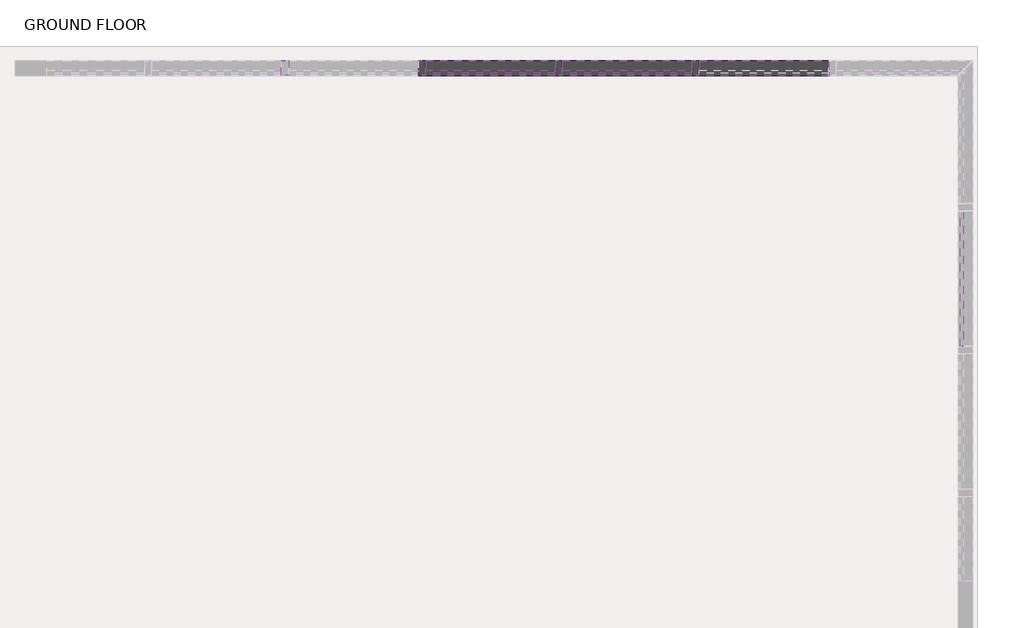
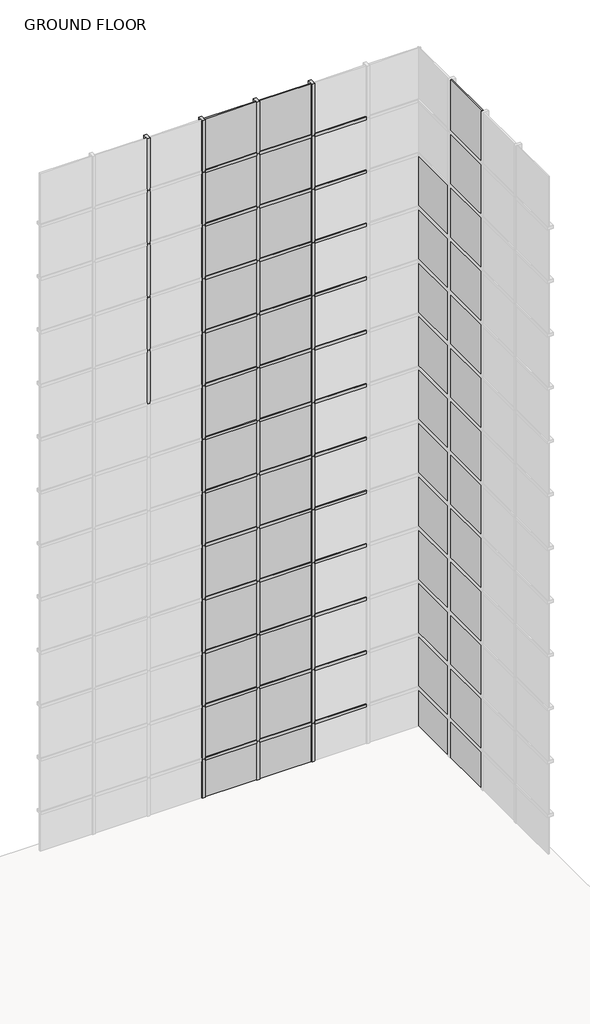
# One storey, part 13 of 16: 80 members, 50 plates.
"""IFC4 building model written with IfcOpenShell, lengths in millimetres."""

from ifc_helpers import new_model, si_unit, origin, place, context, project, spatial, transform, mapped, element, save
from components import member_d518c94e, member_b860638c, member_31fee25f, system_panel_glazed_5cba32e5, system_panel_glazed_49652e9e

model = new_model("IFC4")

# Units and contexts
model_context = context("Model", 3, world=origin())
ifc_project = project(units=[si_unit("LENGTHUNIT", "METRE", prefix="MILLI")], contexts=[model_context])

# Site, building, storey
site = spatial("IfcSite", under=ifc_project)
building = spatial("IfcBuilding", under=site)
storey = spatial("IfcBuildingStorey", under=building, Name="GROUND FLOOR", Elevation=0.0)

# Members
placement = place(None, origin())
member_shape = member_d518c94e(model_context)
element("IfcMember", 1, ObjectType="Rectangular Mullion : 2.5\" x 5\" rectangular", at=placement, inside=storey, context=model_context, shape_type="MappedRepresentation", body=[
    mapped(member_shape, transform((3695.2597848, 6370.2261968, 1168.8884615), x_axis=(0.0, 0.0, 1.0), y_axis=(0.0, 1.0, 0.0), z_axis=(-1.0, 0.0, 0.0))),
])
element("IfcMember", 2, ObjectType="Rectangular Mullion : 2.5\" x 5\" rectangular", at=placement, inside=storey, context=model_context, shape_type="MappedRepresentation", body=[
    mapped(member_shape, transform((2529.7905541, 6370.2261968, 1168.8884615), x_axis=(0.0, 0.0, 1.0), y_axis=(0.0, 1.0, 0.0), z_axis=(-1.0, 0.0, 0.0))),
])
element("IfcMember", 3, ObjectType="Rectangular Mullion : 2.5\" x 5\" rectangular", at=placement, inside=storey, context=model_context, shape_type="MappedRepresentation", body=[
    mapped(member_shape, transform((1364.3213234, 6370.2261968, 1168.8884615), x_axis=(0.0, 0.0, 1.0), y_axis=(0.0, 1.0, 0.0), z_axis=(-1.0, 0.0, 0.0))),
])
element("IfcMember", 4, ObjectType="Rectangular Mullion : 2.5\" x 5\" rectangular", at=placement, inside=storey, context=model_context, shape_type="MappedRepresentation", body=[
    mapped(member_shape, transform((3695.2597848, 6370.2261968, 2369.5269231), x_axis=(0.0, 0.0, 1.0), y_axis=(0.0, 1.0, 0.0), z_axis=(-1.0, 0.0, 0.0))),
])
element("IfcMember", 5, ObjectType="Rectangular Mullion : 2.5\" x 5\" rectangular", at=placement, inside=storey, context=model_context, shape_type="MappedRepresentation", body=[
    mapped(member_shape, transform((2529.7905541, 6370.2261968, 2369.5269231), x_axis=(0.0, 0.0, 1.0), y_axis=(0.0, 1.0, 0.0), z_axis=(-1.0, 0.0, 0.0))),
])
element("IfcMember", 6, ObjectType="Rectangular Mullion : 2.5\" x 5\" rectangular", at=placement, inside=storey, context=model_context, shape_type="MappedRepresentation", body=[
    mapped(member_shape, transform((1364.3213234, 6370.2261968, 2369.5269231), x_axis=(0.0, 0.0, 1.0), y_axis=(0.0, 1.0, 0.0), z_axis=(-1.0, 0.0, 0.0))),
])
element("IfcMember", 7, ObjectType="Rectangular Mullion : 2.5\" x 5\" rectangular", at=placement, inside=storey, context=model_context, shape_type="MappedRepresentation", body=[
    mapped(member_shape, transform((3695.2597848, 6370.2261968, 3570.1653846), x_axis=(0.0, 0.0, 1.0), y_axis=(0.0, 1.0, 0.0), z_axis=(-1.0, 0.0, 0.0))),
])
element("IfcMember", 8, ObjectType="Rectangular Mullion : 2.5\" x 5\" rectangular", at=placement, inside=storey, context=model_context, shape_type="MappedRepresentation", body=[
    mapped(member_shape, transform((2529.7905541, 6370.2261968, 3570.1653846), x_axis=(0.0, 0.0, 1.0), y_axis=(0.0, 1.0, 0.0), z_axis=(-1.0, 0.0, 0.0))),
])
element("IfcMember", 9, ObjectType="Rectangular Mullion : 2.5\" x 5\" rectangular", at=placement, inside=storey, context=model_context, shape_type="MappedRepresentation", body=[
    mapped(member_shape, transform((1364.3213234, 6370.2261968, 3570.1653846), x_axis=(0.0, 0.0, 1.0), y_axis=(0.0, 1.0, 0.0), z_axis=(-1.0, 0.0, 0.0))),
])
element("IfcMember", 10, ObjectType="Rectangular Mullion : 2.5\" x 5\" rectangular", at=placement, inside=storey, context=model_context, shape_type="MappedRepresentation", body=[
    mapped(member_shape, transform((3695.2597848, 6370.2261968, 4770.8038462), x_axis=(0.0, 0.0, 1.0), y_axis=(0.0, 1.0, 0.0), z_axis=(-1.0, 0.0, 0.0))),
])
element("IfcMember", 11, ObjectType="Rectangular Mullion : 2.5\" x 5\" rectangular", at=placement, inside=storey, context=model_context, shape_type="MappedRepresentation", body=[
    mapped(member_shape, transform((2529.7905541, 6370.2261968, 4770.8038462), x_axis=(0.0, 0.0, 1.0), y_axis=(0.0, 1.0, 0.0), z_axis=(-1.0, 0.0, 0.0))),
])
element("IfcMember", 12, ObjectType="Rectangular Mullion : 2.5\" x 5\" rectangular", at=placement, inside=storey, context=model_context, shape_type="MappedRepresentation", body=[
    mapped(member_shape, transform((1364.3213234, 6370.2261968, 4770.8038462), x_axis=(0.0, 0.0, 1.0), y_axis=(0.0, 1.0, 0.0), z_axis=(-1.0, 0.0, 0.0))),
])
element("IfcMember", 13, ObjectType="Rectangular Mullion : 2.5\" x 5\" rectangular", at=placement, inside=storey, context=model_context, shape_type="MappedRepresentation", body=[
    mapped(member_shape, transform((3695.2597848, 6370.2261968, 5971.4423077), x_axis=(0.0, 0.0, 1.0), y_axis=(0.0, 1.0, 0.0), z_axis=(-1.0, 0.0, 0.0))),
])
element("IfcMember", 14, ObjectType="Rectangular Mullion : 2.5\" x 5\" rectangular", at=placement, inside=storey, context=model_context, shape_type="MappedRepresentation", body=[
    mapped(member_shape, transform((2529.7905541, 6370.2261968, 5971.4423077), x_axis=(0.0, 0.0, 1.0), y_axis=(0.0, 1.0, 0.0), z_axis=(-1.0, 0.0, 0.0))),
])
element("IfcMember", 15, ObjectType="Rectangular Mullion : 2.5\" x 5\" rectangular", at=placement, inside=storey, context=model_context, shape_type="MappedRepresentation", body=[
    mapped(member_shape, transform((1364.3213234, 6370.2261968, 5971.4423077), x_axis=(0.0, 0.0, 1.0), y_axis=(0.0, 1.0, 0.0), z_axis=(-1.0, 0.0, 0.0))),
])
element("IfcMember", 16, ObjectType="Rectangular Mullion : 2.5\" x 5\" rectangular", at=placement, inside=storey, context=model_context, shape_type="MappedRepresentation", body=[
    mapped(member_shape, transform((3695.2597848, 6370.2261968, 7172.0807692), x_axis=(0.0, 0.0, 1.0), y_axis=(0.0, 1.0, 0.0), z_axis=(-1.0, 0.0, 0.0))),
])
element("IfcMember", 17, ObjectType="Rectangular Mullion : 2.5\" x 5\" rectangular", at=placement, inside=storey, context=model_context, shape_type="MappedRepresentation", body=[
    mapped(member_shape, transform((2529.7905541, 6370.2261968, 7172.0807692), x_axis=(0.0, 0.0, 1.0), y_axis=(0.0, 1.0, 0.0), z_axis=(-1.0, 0.0, 0.0))),
])
element("IfcMember", 18, ObjectType="Rectangular Mullion : 2.5\" x 5\" rectangular", at=placement, inside=storey, context=model_context, shape_type="MappedRepresentation", body=[
    mapped(member_shape, transform((1364.3213234, 6370.2261968, 7172.0807692), x_axis=(0.0, 0.0, 1.0), y_axis=(0.0, 1.0, 0.0), z_axis=(-1.0, 0.0, 0.0))),
])
element("IfcMember", 19, ObjectType="Rectangular Mullion : 2.5\" x 5\" rectangular", at=placement, inside=storey, context=model_context, shape_type="MappedRepresentation", body=[
    mapped(member_shape, transform((3695.2597848, 6370.2261968, 8372.7192308), x_axis=(0.0, 0.0, 1.0), y_axis=(0.0, 1.0, 0.0), z_axis=(-1.0, 0.0, 0.0))),
])
element("IfcMember", 20, ObjectType="Rectangular Mullion : 2.5\" x 5\" rectangular", at=placement, inside=storey, context=model_context, shape_type="MappedRepresentation", body=[
    mapped(member_shape, transform((2529.7905541, 6370.2261968, 8372.7192308), x_axis=(0.0, 0.0, 1.0), y_axis=(0.0, 1.0, 0.0), z_axis=(-1.0, 0.0, 0.0))),
])
element("IfcMember", 21, ObjectType="Rectangular Mullion : 2.5\" x 5\" rectangular", at=placement, inside=storey, context=model_context, shape_type="MappedRepresentation", body=[
    mapped(member_shape, transform((1364.3213234, 6370.2261968, 8372.7192308), x_axis=(0.0, 0.0, 1.0), y_axis=(0.0, 1.0, 0.0), z_axis=(-1.0, 0.0, 0.0))),
])
element("IfcMember", 22, ObjectType="Rectangular Mullion : 2.5\" x 5\" rectangular", at=placement, inside=storey, context=model_context, shape_type="MappedRepresentation", body=[
    mapped(member_shape, transform((3695.2597848, 6370.2261968, 9573.3576923), x_axis=(0.0, 0.0, 1.0), y_axis=(0.0, 1.0, 0.0), z_axis=(-1.0, 0.0, 0.0))),
])
element("IfcMember", 23, ObjectType="Rectangular Mullion : 2.5\" x 5\" rectangular", at=placement, inside=storey, context=model_context, shape_type="MappedRepresentation", body=[
    mapped(member_shape, transform((2529.7905541, 6370.2261968, 9573.3576923), x_axis=(0.0, 0.0, 1.0), y_axis=(0.0, 1.0, 0.0), z_axis=(-1.0, 0.0, 0.0))),
])
element("IfcMember", 24, ObjectType="Rectangular Mullion : 2.5\" x 5\" rectangular", at=placement, inside=storey, context=model_context, shape_type="MappedRepresentation", body=[
    mapped(member_shape, transform((1364.3213234, 6370.2261968, 9573.3576923), x_axis=(0.0, 0.0, 1.0), y_axis=(0.0, 1.0, 0.0), z_axis=(-1.0, 0.0, 0.0))),
])
element("IfcMember", 25, ObjectType="Rectangular Mullion : 2.5\" x 5\" rectangular", at=placement, inside=storey, context=model_context, shape_type="MappedRepresentation", body=[
    mapped(member_shape, transform((3695.2597848, 6370.2261968, 10773.9961538), x_axis=(0.0, 0.0, 1.0), y_axis=(0.0, 1.0, 0.0), z_axis=(-1.0, 0.0, 0.0))),
])
element("IfcMember", 26, ObjectType="Rectangular Mullion : 2.5\" x 5\" rectangular", at=placement, inside=storey, context=model_context, shape_type="MappedRepresentation", body=[
    mapped(member_shape, transform((2529.7905541, 6370.2261968, 10773.9961538), x_axis=(0.0, 0.0, 1.0), y_axis=(0.0, 1.0, 0.0), z_axis=(-1.0, 0.0, 0.0))),
])
element("IfcMember", 27, ObjectType="Rectangular Mullion : 2.5\" x 5\" rectangular", at=placement, inside=storey, context=model_context, shape_type="MappedRepresentation", body=[
    mapped(member_shape, transform((1364.3213234, 6370.2261968, 10773.9961538), x_axis=(0.0, 0.0, 1.0), y_axis=(0.0, 1.0, 0.0), z_axis=(-1.0, 0.0, 0.0))),
])
element("IfcMember", 28, ObjectType="Rectangular Mullion : 2.5\" x 5\" rectangular", at=placement, inside=storey, context=model_context, shape_type="MappedRepresentation", body=[
    mapped(member_shape, transform((3695.2597848, 6370.2261968, 11974.6346154), x_axis=(0.0, 0.0, 1.0), y_axis=(0.0, 1.0, 0.0), z_axis=(-1.0, 0.0, 0.0))),
])
element("IfcMember", 29, ObjectType="Rectangular Mullion : 2.5\" x 5\" rectangular", at=placement, inside=storey, context=model_context, shape_type="MappedRepresentation", body=[
    mapped(member_shape, transform((2529.7905541, 6370.2261968, 11974.6346154), x_axis=(0.0, 0.0, 1.0), y_axis=(0.0, 1.0, 0.0), z_axis=(-1.0, 0.0, 0.0))),
])
element("IfcMember", 30, ObjectType="Rectangular Mullion : 2.5\" x 5\" rectangular", at=placement, inside=storey, context=model_context, shape_type="MappedRepresentation", body=[
    mapped(member_shape, transform((1364.3213234, 6370.2261968, 11974.6346154), x_axis=(0.0, 0.0, 1.0), y_axis=(0.0, 1.0, 0.0), z_axis=(-1.0, 0.0, 0.0))),
])
element("IfcMember", 31, ObjectType="Rectangular Mullion : 2.5\" x 5\" rectangular", at=placement, inside=storey, context=model_context, shape_type="MappedRepresentation", body=[
    mapped(member_shape, transform((3695.2597848, 6370.2261968, 13175.2730769), x_axis=(0.0, 0.0, 1.0), y_axis=(0.0, 1.0, 0.0), z_axis=(-1.0, 0.0, 0.0))),
])
element("IfcMember", 32, ObjectType="Rectangular Mullion : 2.5\" x 5\" rectangular", at=placement, inside=storey, context=model_context, shape_type="MappedRepresentation", body=[
    mapped(member_shape, transform((2529.7905541, 6370.2261968, 13175.2730769), x_axis=(0.0, 0.0, 1.0), y_axis=(0.0, 1.0, 0.0), z_axis=(-1.0, 0.0, 0.0))),
])
element("IfcMember", 33, ObjectType="Rectangular Mullion : 2.5\" x 5\" rectangular", at=placement, inside=storey, context=model_context, shape_type="MappedRepresentation", body=[
    mapped(member_shape, transform((1364.3213234, 6370.2261968, 13175.2730769), x_axis=(0.0, 0.0, 1.0), y_axis=(0.0, 1.0, 0.0), z_axis=(-1.0, 0.0, 0.0))),
])
element("IfcMember", 34, ObjectType="Rectangular Mullion : 2.5\" x 5\" rectangular", at=placement, inside=storey, context=model_context, shape_type="MappedRepresentation", body=[
    mapped(member_shape, transform((3695.2597848, 6370.2261968, 14375.9115385), x_axis=(0.0, 0.0, 1.0), y_axis=(0.0, 1.0, 0.0), z_axis=(-1.0, 0.0, 0.0))),
])
element("IfcMember", 35, ObjectType="Rectangular Mullion : 2.5\" x 5\" rectangular", at=placement, inside=storey, context=model_context, shape_type="MappedRepresentation", body=[
    mapped(member_shape, transform((2529.7905541, 6370.2261968, 14375.9115385), x_axis=(0.0, 0.0, 1.0), y_axis=(0.0, 1.0, 0.0), z_axis=(-1.0, 0.0, 0.0))),
])
element("IfcMember", 36, ObjectType="Rectangular Mullion : 2.5\" x 5\" rectangular", at=placement, inside=storey, context=model_context, shape_type="MappedRepresentation", body=[
    mapped(member_shape, transform((1364.3213234, 6370.2261968, 14375.9115385), x_axis=(0.0, 0.0, 1.0), y_axis=(0.0, 1.0, 0.0), z_axis=(-1.0, 0.0, 0.0))),
])
member_2_shape = member_b860638c(model_context)
element("IfcMember", 37, ObjectType="Rectangular Mullion : 2.5\" x 5\" rectangular", at=placement, inside=storey, context=model_context, shape_type="MappedRepresentation", body=[
    mapped(member_2_shape, transform((3663.5097848, 6370.2261968, 0.0), x_axis=(-1.0, 0.0, 0.0), y_axis=(0.0, 1.0, 0.0), z_axis=(0.0, 0.0, -1.0))),
])
element("IfcMember", 38, ObjectType="Rectangular Mullion : 2.5\" x 5\" rectangular", at=placement, inside=storey, context=model_context, shape_type="MappedRepresentation", body=[
    mapped(member_2_shape, transform((2498.0405541, 6370.2261968, 0.0), x_axis=(-1.0, 0.0, 0.0), y_axis=(0.0, 1.0, 0.0), z_axis=(0.0, 0.0, -1.0))),
])
element("IfcMember", 39, ObjectType="Rectangular Mullion : 2.5\" x 5\" rectangular", at=placement, inside=storey, context=model_context, shape_type="MappedRepresentation", body=[
    mapped(member_2_shape, transform((1332.5713234, 6370.2261968, 0.0), x_axis=(-1.0, 0.0, 0.0), y_axis=(0.0, 1.0, 0.0), z_axis=(0.0, 0.0, -1.0))),
])
member_3_shape = member_31fee25f(model_context)
element("IfcMember", 40, ObjectType="Rectangular Mullion : 2.5\" x 5\" rectangular", at=placement, inside=storey, context=model_context, shape_type="MappedRepresentation", body=[
    mapped(member_3_shape, transform((3663.5097848, 6370.2261968, 1168.8884615), x_axis=(-1.0, 0.0, 0.0), y_axis=(0.0, 1.0, 0.0), z_axis=(0.0, 0.0, -1.0))),
])
element("IfcMember", 41, ObjectType="Rectangular Mullion : 2.5\" x 5\" rectangular", at=placement, inside=storey, context=model_context, shape_type="MappedRepresentation", body=[
    mapped(member_3_shape, transform((2498.0405541, 6370.2261968, 1168.8884615), x_axis=(-1.0, 0.0, 0.0), y_axis=(0.0, 1.0, 0.0), z_axis=(0.0, 0.0, -1.0))),
])
element("IfcMember", 42, ObjectType="Rectangular Mullion : 2.5\" x 5\" rectangular", at=placement, inside=storey, context=model_context, shape_type="MappedRepresentation", body=[
    mapped(member_3_shape, transform((1332.5713234, 6370.2261968, 1168.8884615), x_axis=(-1.0, 0.0, 0.0), y_axis=(0.0, 1.0, 0.0), z_axis=(0.0, 0.0, -1.0))),
])
element("IfcMember", 43, ObjectType="Rectangular Mullion : 2.5\" x 5\" rectangular", at=placement, inside=storey, context=model_context, shape_type="MappedRepresentation", body=[
    mapped(member_3_shape, transform((3663.5097848, 6370.2261968, 2369.5269231), x_axis=(-1.0, 0.0, 0.0), y_axis=(0.0, 1.0, 0.0), z_axis=(0.0, 0.0, -1.0))),
])
element("IfcMember", 44, ObjectType="Rectangular Mullion : 2.5\" x 5\" rectangular", at=placement, inside=storey, context=model_context, shape_type="MappedRepresentation", body=[
    mapped(member_3_shape, transform((2498.0405541, 6370.2261968, 2369.5269231), x_axis=(-1.0, 0.0, 0.0), y_axis=(0.0, 1.0, 0.0), z_axis=(0.0, 0.0, -1.0))),
])
element("IfcMember", 45, ObjectType="Rectangular Mullion : 2.5\" x 5\" rectangular", at=placement, inside=storey, context=model_context, shape_type="MappedRepresentation", body=[
    mapped(member_3_shape, transform((1332.5713234, 6370.2261968, 2369.5269231), x_axis=(-1.0, 0.0, 0.0), y_axis=(0.0, 1.0, 0.0), z_axis=(0.0, 0.0, -1.0))),
])
element("IfcMember", 46, ObjectType="Rectangular Mullion : 2.5\" x 5\" rectangular", at=placement, inside=storey, context=model_context, shape_type="MappedRepresentation", body=[
    mapped(member_3_shape, transform((3663.5097848, 6370.2261968, 3570.1653846), x_axis=(-1.0, 0.0, 0.0), y_axis=(0.0, 1.0, 0.0), z_axis=(0.0, 0.0, -1.0))),
])
element("IfcMember", 47, ObjectType="Rectangular Mullion : 2.5\" x 5\" rectangular", at=placement, inside=storey, context=model_context, shape_type="MappedRepresentation", body=[
    mapped(member_3_shape, transform((2498.0405541, 6370.2261968, 3570.1653846), x_axis=(-1.0, 0.0, 0.0), y_axis=(0.0, 1.0, 0.0), z_axis=(0.0, 0.0, -1.0))),
])
element("IfcMember", 48, ObjectType="Rectangular Mullion : 2.5\" x 5\" rectangular", at=placement, inside=storey, context=model_context, shape_type="MappedRepresentation", body=[
    mapped(member_3_shape, transform((1332.5713234, 6370.2261968, 3570.1653846), x_axis=(-1.0, 0.0, 0.0), y_axis=(0.0, 1.0, 0.0), z_axis=(0.0, 0.0, -1.0))),
])
element("IfcMember", 49, ObjectType="Rectangular Mullion : 2.5\" x 5\" rectangular", at=placement, inside=storey, context=model_context, shape_type="MappedRepresentation", body=[
    mapped(member_3_shape, transform((3663.5097848, 6370.2261968, 4770.8038462), x_axis=(-1.0, 0.0, 0.0), y_axis=(0.0, 1.0, 0.0), z_axis=(0.0, 0.0, -1.0))),
])
element("IfcMember", 50, ObjectType="Rectangular Mullion : 2.5\" x 5\" rectangular", at=placement, inside=storey, context=model_context, shape_type="MappedRepresentation", body=[
    mapped(member_3_shape, transform((2498.0405541, 6370.2261968, 4770.8038462), x_axis=(-1.0, 0.0, 0.0), y_axis=(0.0, 1.0, 0.0), z_axis=(0.0, 0.0, -1.0))),
])
element("IfcMember", 51, ObjectType="Rectangular Mullion : 2.5\" x 5\" rectangular", at=placement, inside=storey, context=model_context, shape_type="MappedRepresentation", body=[
    mapped(member_3_shape, transform((1332.5713234, 6370.2261968, 4770.8038462), x_axis=(-1.0, 0.0, 0.0), y_axis=(0.0, 1.0, 0.0), z_axis=(0.0, 0.0, -1.0))),
])
element("IfcMember", 52, ObjectType="Rectangular Mullion : 2.5\" x 5\" rectangular", at=placement, inside=storey, context=model_context, shape_type="MappedRepresentation", body=[
    mapped(member_3_shape, transform((3663.5097848, 6370.2261968, 5971.4423077), x_axis=(-1.0, 0.0, 0.0), y_axis=(0.0, 1.0, 0.0), z_axis=(0.0, 0.0, -1.0))),
])
element("IfcMember", 53, ObjectType="Rectangular Mullion : 2.5\" x 5\" rectangular", at=placement, inside=storey, context=model_context, shape_type="MappedRepresentation", body=[
    mapped(member_3_shape, transform((2498.0405541, 6370.2261968, 5971.4423077), x_axis=(-1.0, 0.0, 0.0), y_axis=(0.0, 1.0, 0.0), z_axis=(0.0, 0.0, -1.0))),
])
element("IfcMember", 54, ObjectType="Rectangular Mullion : 2.5\" x 5\" rectangular", at=placement, inside=storey, context=model_context, shape_type="MappedRepresentation", body=[
    mapped(member_3_shape, transform((1332.5713234, 6370.2261968, 5971.4423077), x_axis=(-1.0, 0.0, 0.0), y_axis=(0.0, 1.0, 0.0), z_axis=(0.0, 0.0, -1.0))),
])
element("IfcMember", 55, ObjectType="Rectangular Mullion : 2.5\" x 5\" rectangular", at=placement, inside=storey, context=model_context, shape_type="MappedRepresentation", body=[
    mapped(member_3_shape, transform((3663.5097848, 6370.2261968, 7172.0807692), x_axis=(-1.0, 0.0, 0.0), y_axis=(0.0, 1.0, 0.0), z_axis=(0.0, 0.0, -1.0))),
])
element("IfcMember", 56, ObjectType="Rectangular Mullion : 2.5\" x 5\" rectangular", at=placement, inside=storey, context=model_context, shape_type="MappedRepresentation", body=[
    mapped(member_3_shape, transform((2498.0405541, 6370.2261968, 7172.0807692), x_axis=(-1.0, 0.0, 0.0), y_axis=(0.0, 1.0, 0.0), z_axis=(0.0, 0.0, -1.0))),
])
element("IfcMember", 57, ObjectType="Rectangular Mullion : 2.5\" x 5\" rectangular", at=placement, inside=storey, context=model_context, shape_type="MappedRepresentation", body=[
    mapped(member_3_shape, transform((1332.5713234, 6370.2261968, 7172.0807692), x_axis=(-1.0, 0.0, 0.0), y_axis=(0.0, 1.0, 0.0), z_axis=(0.0, 0.0, -1.0))),
])
element("IfcMember", 58, ObjectType="Rectangular Mullion : 2.5\" x 5\" rectangular", at=placement, inside=storey, context=model_context, shape_type="MappedRepresentation", body=[
    mapped(member_3_shape, transform((3663.5097848, 6370.2261968, 8372.7192308), x_axis=(-1.0, 0.0, 0.0), y_axis=(0.0, 1.0, 0.0), z_axis=(0.0, 0.0, -1.0))),
])
element("IfcMember", 59, ObjectType="Rectangular Mullion : 2.5\" x 5\" rectangular", at=placement, inside=storey, context=model_context, shape_type="MappedRepresentation", body=[
    mapped(member_3_shape, transform((2498.0405541, 6370.2261968, 8372.7192308), x_axis=(-1.0, 0.0, 0.0), y_axis=(0.0, 1.0, 0.0), z_axis=(0.0, 0.0, -1.0))),
])
element("IfcMember", 60, ObjectType="Rectangular Mullion : 2.5\" x 5\" rectangular", at=placement, inside=storey, context=model_context, shape_type="MappedRepresentation", body=[
    mapped(member_3_shape, transform((1332.5713234, 6370.2261968, 8372.7192308), x_axis=(-1.0, 0.0, 0.0), y_axis=(0.0, 1.0, 0.0), z_axis=(0.0, 0.0, -1.0))),
])
element("IfcMember", 61, ObjectType="Rectangular Mullion : 2.5\" x 5\" rectangular", at=placement, inside=storey, context=model_context, shape_type="MappedRepresentation", body=[
    mapped(member_3_shape, transform((3663.5097848, 6370.2261968, 9573.3576923), x_axis=(-1.0, 0.0, 0.0), y_axis=(0.0, 1.0, 0.0), z_axis=(0.0, 0.0, -1.0))),
])
element("IfcMember", 62, ObjectType="Rectangular Mullion : 2.5\" x 5\" rectangular", at=placement, inside=storey, context=model_context, shape_type="MappedRepresentation", body=[
    mapped(member_3_shape, transform((2498.0405541, 6370.2261968, 9573.3576923), x_axis=(-1.0, 0.0, 0.0), y_axis=(0.0, 1.0, 0.0), z_axis=(0.0, 0.0, -1.0))),
])
element("IfcMember", 63, ObjectType="Rectangular Mullion : 2.5\" x 5\" rectangular", at=placement, inside=storey, context=model_context, shape_type="MappedRepresentation", body=[
    mapped(member_3_shape, transform((1332.5713234, 6370.2261968, 9573.3576923), x_axis=(-1.0, 0.0, 0.0), y_axis=(0.0, 1.0, 0.0), z_axis=(0.0, 0.0, -1.0))),
])
element("IfcMember", 64, ObjectType="Rectangular Mullion : 2.5\" x 5\" rectangular", at=placement, inside=storey, context=model_context, shape_type="MappedRepresentation", body=[
    mapped(member_3_shape, transform((167.1020927, 6370.2261968, 9573.3576923), x_axis=(-1.0, 0.0, 0.0), y_axis=(0.0, 1.0, 0.0), z_axis=(0.0, 0.0, -1.0))),
])
element("IfcMember", 65, ObjectType="Rectangular Mullion : 2.5\" x 5\" rectangular", at=placement, inside=storey, context=model_context, shape_type="MappedRepresentation", body=[
    mapped(member_3_shape, transform((3663.5097848, 6370.2261968, 10773.9961538), x_axis=(-1.0, 0.0, 0.0), y_axis=(0.0, 1.0, 0.0), z_axis=(0.0, 0.0, -1.0))),
])
element("IfcMember", 66, ObjectType="Rectangular Mullion : 2.5\" x 5\" rectangular", at=placement, inside=storey, context=model_context, shape_type="MappedRepresentation", body=[
    mapped(member_3_shape, transform((2498.0405541, 6370.2261968, 10773.9961538), x_axis=(-1.0, 0.0, 0.0), y_axis=(0.0, 1.0, 0.0), z_axis=(0.0, 0.0, -1.0))),
])
element("IfcMember", 67, ObjectType="Rectangular Mullion : 2.5\" x 5\" rectangular", at=placement, inside=storey, context=model_context, shape_type="MappedRepresentation", body=[
    mapped(member_3_shape, transform((1332.5713234, 6370.2261968, 10773.9961538), x_axis=(-1.0, 0.0, 0.0), y_axis=(0.0, 1.0, 0.0), z_axis=(0.0, 0.0, -1.0))),
])
element("IfcMember", 68, ObjectType="Rectangular Mullion : 2.5\" x 5\" rectangular", at=placement, inside=storey, context=model_context, shape_type="MappedRepresentation", body=[
    mapped(member_3_shape, transform((167.1020927, 6370.2261968, 10773.9961538), x_axis=(-1.0, 0.0, 0.0), y_axis=(0.0, 1.0, 0.0), z_axis=(0.0, 0.0, -1.0))),
])
element("IfcMember", 69, ObjectType="Rectangular Mullion : 2.5\" x 5\" rectangular", at=placement, inside=storey, context=model_context, shape_type="MappedRepresentation", body=[
    mapped(member_3_shape, transform((3663.5097848, 6370.2261968, 11974.6346154), x_axis=(-1.0, 0.0, 0.0), y_axis=(0.0, 1.0, 0.0), z_axis=(0.0, 0.0, -1.0))),
])
element("IfcMember", 70, ObjectType="Rectangular Mullion : 2.5\" x 5\" rectangular", at=placement, inside=storey, context=model_context, shape_type="MappedRepresentation", body=[
    mapped(member_3_shape, transform((2498.0405541, 6370.2261968, 11974.6346154), x_axis=(-1.0, 0.0, 0.0), y_axis=(0.0, 1.0, 0.0), z_axis=(0.0, 0.0, -1.0))),
])
element("IfcMember", 71, ObjectType="Rectangular Mullion : 2.5\" x 5\" rectangular", at=placement, inside=storey, context=model_context, shape_type="MappedRepresentation", body=[
    mapped(member_3_shape, transform((1332.5713234, 6370.2261968, 11974.6346154), x_axis=(-1.0, 0.0, 0.0), y_axis=(0.0, 1.0, 0.0), z_axis=(0.0, 0.0, -1.0))),
])
element("IfcMember", 72, ObjectType="Rectangular Mullion : 2.5\" x 5\" rectangular", at=placement, inside=storey, context=model_context, shape_type="MappedRepresentation", body=[
    mapped(member_3_shape, transform((167.1020927, 6370.2261968, 11974.6346154), x_axis=(-1.0, 0.0, 0.0), y_axis=(0.0, 1.0, 0.0), z_axis=(0.0, 0.0, -1.0))),
])
element("IfcMember", 73, ObjectType="Rectangular Mullion : 2.5\" x 5\" rectangular", at=placement, inside=storey, context=model_context, shape_type="MappedRepresentation", body=[
    mapped(member_3_shape, transform((3663.5097848, 6370.2261968, 13175.2730769), x_axis=(-1.0, 0.0, 0.0), y_axis=(0.0, 1.0, 0.0), z_axis=(0.0, 0.0, -1.0))),
])
element("IfcMember", 74, ObjectType="Rectangular Mullion : 2.5\" x 5\" rectangular", at=placement, inside=storey, context=model_context, shape_type="MappedRepresentation", body=[
    mapped(member_3_shape, transform((2498.0405541, 6370.2261968, 13175.2730769), x_axis=(-1.0, 0.0, 0.0), y_axis=(0.0, 1.0, 0.0), z_axis=(0.0, 0.0, -1.0))),
])
element("IfcMember", 75, ObjectType="Rectangular Mullion : 2.5\" x 5\" rectangular", at=placement, inside=storey, context=model_context, shape_type="MappedRepresentation", body=[
    mapped(member_3_shape, transform((1332.5713234, 6370.2261968, 13175.2730769), x_axis=(-1.0, 0.0, 0.0), y_axis=(0.0, 1.0, 0.0), z_axis=(0.0, 0.0, -1.0))),
])
element("IfcMember", 76, ObjectType="Rectangular Mullion : 2.5\" x 5\" rectangular", at=placement, inside=storey, context=model_context, shape_type="MappedRepresentation", body=[
    mapped(member_3_shape, transform((167.1020927, 6370.2261968, 13175.2730769), x_axis=(-1.0, 0.0, 0.0), y_axis=(0.0, 1.0, 0.0), z_axis=(0.0, 0.0, -1.0))),
])
element("IfcMember", 77, ObjectType="Rectangular Mullion : 2.5\" x 5\" rectangular", at=placement, inside=storey, context=model_context, shape_type="MappedRepresentation", body=[
    mapped(member_2_shape, transform((3663.5097848, 6370.2261968, 14375.9115385), x_axis=(-1.0, 0.0, 0.0), y_axis=(0.0, 1.0, 0.0), z_axis=(0.0, 0.0, -1.0))),
])
element("IfcMember", 78, ObjectType="Rectangular Mullion : 2.5\" x 5\" rectangular", at=placement, inside=storey, context=model_context, shape_type="MappedRepresentation", body=[
    mapped(member_2_shape, transform((2498.0405541, 6370.2261968, 14375.9115385), x_axis=(-1.0, 0.0, 0.0), y_axis=(0.0, 1.0, 0.0), z_axis=(0.0, 0.0, -1.0))),
])
element("IfcMember", 79, ObjectType="Rectangular Mullion : 2.5\" x 5\" rectangular", at=placement, inside=storey, context=model_context, shape_type="MappedRepresentation", body=[
    mapped(member_2_shape, transform((1332.5713234, 6370.2261968, 14375.9115385), x_axis=(-1.0, 0.0, 0.0), y_axis=(0.0, 1.0, 0.0), z_axis=(0.0, 0.0, -1.0))),
])
element("IfcMember", 80, ObjectType="Rectangular Mullion : 2.5\" x 5\" rectangular", at=placement, inside=storey, context=model_context, shape_type="MappedRepresentation", body=[
    mapped(member_2_shape, transform((167.1020927, 6370.2261968, 14375.9115385), x_axis=(-1.0, 0.0, 0.0), y_axis=(0.0, 1.0, 0.0), z_axis=(0.0, 0.0, -1.0))),
])

# Plates
system_panel_glazed_shape = system_panel_glazed_5cba32e5(model_context)
element("IfcPlate", 81, ObjectType="System Panel : Glazed", at=placement, inside=storey, context=model_context, shape_type="MappedRepresentation", body=[
    mapped(system_panel_glazed_shape, transform((3080.7751695, 6370.2261968, 0.0), x_axis=(-1.0, 0.0, 0.0), y_axis=(0.0, -1.0, 0.0), z_axis=(0.0, 0.0, 1.0))),
])
element("IfcPlate", 82, ObjectType="System Panel : Glazed", at=placement, inside=storey, context=model_context, shape_type="MappedRepresentation", body=[
    mapped(system_panel_glazed_shape, transform((1915.3059387, 6370.2261968, 0.0), x_axis=(-1.0, 0.0, 0.0), y_axis=(0.0, -1.0, 0.0), z_axis=(0.0, 0.0, 1.0))),
])
element("IfcPlate", 83, ObjectType="System Panel : Glazed", at=placement, inside=storey, context=model_context, shape_type="MappedRepresentation", body=[
    mapped(system_panel_glazed_shape, transform((3080.7751695, 6370.2261968, 1200.6384615), x_axis=(-1.0, 0.0, 0.0), y_axis=(0.0, -1.0, 0.0), z_axis=(0.0, 0.0, 1.0))),
])
element("IfcPlate", 84, ObjectType="System Panel : Glazed", at=placement, inside=storey, context=model_context, shape_type="MappedRepresentation", body=[
    mapped(system_panel_glazed_shape, transform((1915.3059387, 6370.2261968, 1200.6384615), x_axis=(-1.0, 0.0, 0.0), y_axis=(0.0, -1.0, 0.0), z_axis=(0.0, 0.0, 1.0))),
])
element("IfcPlate", 85, ObjectType="System Panel : Glazed", at=placement, inside=storey, context=model_context, shape_type="MappedRepresentation", body=[
    mapped(system_panel_glazed_shape, transform((3080.7751695, 6370.2261968, 2401.2769231), x_axis=(-1.0, 0.0, 0.0), y_axis=(0.0, -1.0, 0.0), z_axis=(0.0, 0.0, 1.0))),
])
element("IfcPlate", 86, ObjectType="System Panel : Glazed", at=placement, inside=storey, context=model_context, shape_type="MappedRepresentation", body=[
    mapped(system_panel_glazed_shape, transform((1915.3059387, 6370.2261968, 2401.2769231), x_axis=(-1.0, 0.0, 0.0), y_axis=(0.0, -1.0, 0.0), z_axis=(0.0, 0.0, 1.0))),
])
element("IfcPlate", 87, ObjectType="System Panel : Glazed", at=placement, inside=storey, context=model_context, shape_type="MappedRepresentation", body=[
    mapped(system_panel_glazed_shape, transform((3080.7751695, 6370.2261968, 3601.9153846), x_axis=(-1.0, 0.0, 0.0), y_axis=(0.0, -1.0, 0.0), z_axis=(0.0, 0.0, 1.0))),
])
element("IfcPlate", 88, ObjectType="System Panel : Glazed", at=placement, inside=storey, context=model_context, shape_type="MappedRepresentation", body=[
    mapped(system_panel_glazed_shape, transform((1915.3059387, 6370.2261968, 3601.9153846), x_axis=(-1.0, 0.0, 0.0), y_axis=(0.0, -1.0, 0.0), z_axis=(0.0, 0.0, 1.0))),
])
element("IfcPlate", 89, ObjectType="System Panel : Glazed", at=placement, inside=storey, context=model_context, shape_type="MappedRepresentation", body=[
    mapped(system_panel_glazed_shape, transform((3080.7751695, 6370.2261968, 4802.5538462), x_axis=(-1.0, 0.0, 0.0), y_axis=(0.0, -1.0, 0.0), z_axis=(0.0, 0.0, 1.0))),
])
element("IfcPlate", 90, ObjectType="System Panel : Glazed", at=placement, inside=storey, context=model_context, shape_type="MappedRepresentation", body=[
    mapped(system_panel_glazed_shape, transform((1915.3059387, 6370.2261968, 4802.5538462), x_axis=(-1.0, 0.0, 0.0), y_axis=(0.0, -1.0, 0.0), z_axis=(0.0, 0.0, 1.0))),
])
element("IfcPlate", 91, ObjectType="System Panel : Glazed", at=placement, inside=storey, context=model_context, shape_type="MappedRepresentation", body=[
    mapped(system_panel_glazed_shape, transform((3080.7751695, 6370.2261968, 6003.1923077), x_axis=(-1.0, 0.0, 0.0), y_axis=(0.0, -1.0, 0.0), z_axis=(0.0, 0.0, 1.0))),
])
element("IfcPlate", 92, ObjectType="System Panel : Glazed", at=placement, inside=storey, context=model_context, shape_type="MappedRepresentation", body=[
    mapped(system_panel_glazed_shape, transform((1915.3059387, 6370.2261968, 6003.1923077), x_axis=(-1.0, 0.0, 0.0), y_axis=(0.0, -1.0, 0.0), z_axis=(0.0, 0.0, 1.0))),
])
element("IfcPlate", 93, ObjectType="System Panel : Glazed", at=placement, inside=storey, context=model_context, shape_type="MappedRepresentation", body=[
    mapped(system_panel_glazed_shape, transform((3080.7751695, 6370.2261968, 7203.8307692), x_axis=(-1.0, 0.0, 0.0), y_axis=(0.0, -1.0, 0.0), z_axis=(0.0, 0.0, 1.0))),
])
element("IfcPlate", 94, ObjectType="System Panel : Glazed", at=placement, inside=storey, context=model_context, shape_type="MappedRepresentation", body=[
    mapped(system_panel_glazed_shape, transform((1915.3059387, 6370.2261968, 7203.8307692), x_axis=(-1.0, 0.0, 0.0), y_axis=(0.0, -1.0, 0.0), z_axis=(0.0, 0.0, 1.0))),
])
element("IfcPlate", 95, ObjectType="System Panel : Glazed", at=placement, inside=storey, context=model_context, shape_type="MappedRepresentation", body=[
    mapped(system_panel_glazed_shape, transform((3080.7751695, 6370.2261968, 8404.4692308), x_axis=(-1.0, 0.0, 0.0), y_axis=(0.0, -1.0, 0.0), z_axis=(0.0, 0.0, 1.0))),
])
element("IfcPlate", 96, ObjectType="System Panel : Glazed", at=placement, inside=storey, context=model_context, shape_type="MappedRepresentation", body=[
    mapped(system_panel_glazed_shape, transform((1915.3059387, 6370.2261968, 8404.4692308), x_axis=(-1.0, 0.0, 0.0), y_axis=(0.0, -1.0, 0.0), z_axis=(0.0, 0.0, 1.0))),
])
element("IfcPlate", 97, ObjectType="System Panel : Glazed", at=placement, inside=storey, context=model_context, shape_type="MappedRepresentation", body=[
    mapped(system_panel_glazed_shape, transform((3080.7751695, 6370.2261968, 9605.1076923), x_axis=(-1.0, 0.0, 0.0), y_axis=(0.0, -1.0, 0.0), z_axis=(0.0, 0.0, 1.0))),
])
element("IfcPlate", 98, ObjectType="System Panel : Glazed", at=placement, inside=storey, context=model_context, shape_type="MappedRepresentation", body=[
    mapped(system_panel_glazed_shape, transform((1915.3059387, 6370.2261968, 9605.1076923), x_axis=(-1.0, 0.0, 0.0), y_axis=(0.0, -1.0, 0.0), z_axis=(0.0, 0.0, 1.0))),
])
element("IfcPlate", 99, ObjectType="System Panel : Glazed", at=placement, inside=storey, context=model_context, shape_type="MappedRepresentation", body=[
    mapped(system_panel_glazed_shape, transform((3080.7751695, 6370.2261968, 10805.7461538), x_axis=(-1.0, 0.0, 0.0), y_axis=(0.0, -1.0, 0.0), z_axis=(0.0, 0.0, 1.0))),
])
element("IfcPlate", 100, ObjectType="System Panel : Glazed", at=placement, inside=storey, context=model_context, shape_type="MappedRepresentation", body=[
    mapped(system_panel_glazed_shape, transform((1915.3059387, 6370.2261968, 10805.7461538), x_axis=(-1.0, 0.0, 0.0), y_axis=(0.0, -1.0, 0.0), z_axis=(0.0, 0.0, 1.0))),
])
element("IfcPlate", 101, ObjectType="System Panel : Glazed", at=placement, inside=storey, context=model_context, shape_type="MappedRepresentation", body=[
    mapped(system_panel_glazed_shape, transform((3080.7751695, 6370.2261968, 12006.3846154), x_axis=(-1.0, 0.0, 0.0), y_axis=(0.0, -1.0, 0.0), z_axis=(0.0, 0.0, 1.0))),
])
element("IfcPlate", 102, ObjectType="System Panel : Glazed", at=placement, inside=storey, context=model_context, shape_type="MappedRepresentation", body=[
    mapped(system_panel_glazed_shape, transform((1915.3059387, 6370.2261968, 12006.3846154), x_axis=(-1.0, 0.0, 0.0), y_axis=(0.0, -1.0, 0.0), z_axis=(0.0, 0.0, 1.0))),
])
element("IfcPlate", 103, ObjectType="System Panel : Glazed", at=placement, inside=storey, context=model_context, shape_type="MappedRepresentation", body=[
    mapped(system_panel_glazed_shape, transform((3080.7751695, 6370.2261968, 13207.0230769), x_axis=(-1.0, 0.0, 0.0), y_axis=(0.0, -1.0, 0.0), z_axis=(0.0, 0.0, 1.0))),
])
element("IfcPlate", 104, ObjectType="System Panel : Glazed", at=placement, inside=storey, context=model_context, shape_type="MappedRepresentation", body=[
    mapped(system_panel_glazed_shape, transform((1915.3059387, 6370.2261968, 13207.0230769), x_axis=(-1.0, 0.0, 0.0), y_axis=(0.0, -1.0, 0.0), z_axis=(0.0, 0.0, 1.0))),
])
element("IfcPlate", 105, ObjectType="System Panel : Glazed", at=placement, inside=storey, context=model_context, shape_type="MappedRepresentation", body=[
    mapped(system_panel_glazed_shape, transform((3080.7751695, 6370.2261968, 14407.6615385), x_axis=(-1.0, 0.0, 0.0), y_axis=(0.0, -1.0, 0.0), z_axis=(0.0, 0.0, 1.0))),
])
element("IfcPlate", 106, ObjectType="System Panel : Glazed", at=placement, inside=storey, context=model_context, shape_type="MappedRepresentation", body=[
    mapped(system_panel_glazed_shape, transform((1915.3059387, 6370.2261968, 14407.6615385), x_axis=(-1.0, 0.0, 0.0), y_axis=(0.0, -1.0, 0.0), z_axis=(0.0, 0.0, 1.0))),
])
system_panel_glazed_2_shape = system_panel_glazed_49652e9e(model_context)
element("IfcPlate", 107, ObjectType="System Panel : Glazed", at=placement, inside=storey, context=model_context, shape_type="MappedRepresentation", body=[
    mapped(system_panel_glazed_2_shape, transform((5962.6982466, 4576.0336966, 0.0), x_axis=(0.0, 1.0, 0.0), y_axis=(-1.0, 0.0, 0.0), z_axis=(0.0, 0.0, 1.0))),
])
element("IfcPlate", 108, ObjectType="System Panel : Glazed", at=placement, inside=storey, context=model_context, shape_type="MappedRepresentation", body=[
    mapped(system_panel_glazed_2_shape, transform((5962.6982466, 5793.3286967, 0.0), x_axis=(0.0, 1.0, 0.0), y_axis=(-1.0, 0.0, 0.0), z_axis=(0.0, 0.0, 1.0))),
])
element("IfcPlate", 109, ObjectType="System Panel : Glazed", at=placement, inside=storey, context=model_context, shape_type="MappedRepresentation", body=[
    mapped(system_panel_glazed_2_shape, transform((5962.6982466, 4576.0336966, 1200.6384615), x_axis=(0.0, 1.0, 0.0), y_axis=(-1.0, 0.0, 0.0), z_axis=(0.0, 0.0, 1.0))),
])
element("IfcPlate", 110, ObjectType="System Panel : Glazed", at=placement, inside=storey, context=model_context, shape_type="MappedRepresentation", body=[
    mapped(system_panel_glazed_2_shape, transform((5962.6982466, 5793.3286967, 1200.6384615), x_axis=(0.0, 1.0, 0.0), y_axis=(-1.0, 0.0, 0.0), z_axis=(0.0, 0.0, 1.0))),
])
element("IfcPlate", 111, ObjectType="System Panel : Glazed", at=placement, inside=storey, context=model_context, shape_type="MappedRepresentation", body=[
    mapped(system_panel_glazed_2_shape, transform((5962.6982466, 4576.0336966, 2401.2769231), x_axis=(0.0, 1.0, 0.0), y_axis=(-1.0, 0.0, 0.0), z_axis=(0.0, 0.0, 1.0))),
])
element("IfcPlate", 112, ObjectType="System Panel : Glazed", at=placement, inside=storey, context=model_context, shape_type="MappedRepresentation", body=[
    mapped(system_panel_glazed_2_shape, transform((5962.6982466, 5793.3286967, 2401.2769231), x_axis=(0.0, 1.0, 0.0), y_axis=(-1.0, 0.0, 0.0), z_axis=(0.0, 0.0, 1.0))),
])
element("IfcPlate", 113, ObjectType="System Panel : Glazed", at=placement, inside=storey, context=model_context, shape_type="MappedRepresentation", body=[
    mapped(system_panel_glazed_2_shape, transform((5962.6982466, 4576.0336966, 3601.9153846), x_axis=(0.0, 1.0, 0.0), y_axis=(-1.0, 0.0, 0.0), z_axis=(0.0, 0.0, 1.0))),
])
element("IfcPlate", 114, ObjectType="System Panel : Glazed", at=placement, inside=storey, context=model_context, shape_type="MappedRepresentation", body=[
    mapped(system_panel_glazed_2_shape, transform((5962.6982466, 5793.3286967, 3601.9153846), x_axis=(0.0, 1.0, 0.0), y_axis=(-1.0, 0.0, 0.0), z_axis=(0.0, 0.0, 1.0))),
])
element("IfcPlate", 115, ObjectType="System Panel : Glazed", at=placement, inside=storey, context=model_context, shape_type="MappedRepresentation", body=[
    mapped(system_panel_glazed_2_shape, transform((5962.6982466, 4576.0336966, 4802.5538462), x_axis=(0.0, 1.0, 0.0), y_axis=(-1.0, 0.0, 0.0), z_axis=(0.0, 0.0, 1.0))),
])
element("IfcPlate", 116, ObjectType="System Panel : Glazed", at=placement, inside=storey, context=model_context, shape_type="MappedRepresentation", body=[
    mapped(system_panel_glazed_2_shape, transform((5962.6982466, 5793.3286967, 4802.5538462), x_axis=(0.0, 1.0, 0.0), y_axis=(-1.0, 0.0, 0.0), z_axis=(0.0, 0.0, 1.0))),
])
element("IfcPlate", 117, ObjectType="System Panel : Glazed", at=placement, inside=storey, context=model_context, shape_type="MappedRepresentation", body=[
    mapped(system_panel_glazed_2_shape, transform((5962.6982466, 4576.0336966, 6003.1923077), x_axis=(0.0, 1.0, 0.0), y_axis=(-1.0, 0.0, 0.0), z_axis=(0.0, 0.0, 1.0))),
])
element("IfcPlate", 118, ObjectType="System Panel : Glazed", at=placement, inside=storey, context=model_context, shape_type="MappedRepresentation", body=[
    mapped(system_panel_glazed_2_shape, transform((5962.6982466, 5793.3286967, 6003.1923077), x_axis=(0.0, 1.0, 0.0), y_axis=(-1.0, 0.0, 0.0), z_axis=(0.0, 0.0, 1.0))),
])
element("IfcPlate", 119, ObjectType="System Panel : Glazed", at=placement, inside=storey, context=model_context, shape_type="MappedRepresentation", body=[
    mapped(system_panel_glazed_2_shape, transform((5962.6982466, 4576.0336966, 7203.8307692), x_axis=(0.0, 1.0, 0.0), y_axis=(-1.0, 0.0, 0.0), z_axis=(0.0, 0.0, 1.0))),
])
element("IfcPlate", 120, ObjectType="System Panel : Glazed", at=placement, inside=storey, context=model_context, shape_type="MappedRepresentation", body=[
    mapped(system_panel_glazed_2_shape, transform((5962.6982466, 5793.3286967, 7203.8307692), x_axis=(0.0, 1.0, 0.0), y_axis=(-1.0, 0.0, 0.0), z_axis=(0.0, 0.0, 1.0))),
])
element("IfcPlate", 121, ObjectType="System Panel : Glazed", at=placement, inside=storey, context=model_context, shape_type="MappedRepresentation", body=[
    mapped(system_panel_glazed_2_shape, transform((5962.6982466, 4576.0336966, 8404.4692308), x_axis=(0.0, 1.0, 0.0), y_axis=(-1.0, 0.0, 0.0), z_axis=(0.0, 0.0, 1.0))),
])
element("IfcPlate", 122, ObjectType="System Panel : Glazed", at=placement, inside=storey, context=model_context, shape_type="MappedRepresentation", body=[
    mapped(system_panel_glazed_2_shape, transform((5962.6982466, 5793.3286967, 8404.4692308), x_axis=(0.0, 1.0, 0.0), y_axis=(-1.0, 0.0, 0.0), z_axis=(0.0, 0.0, 1.0))),
])
element("IfcPlate", 123, ObjectType="System Panel : Glazed", at=placement, inside=storey, context=model_context, shape_type="MappedRepresentation", body=[
    mapped(system_panel_glazed_2_shape, transform((5962.6982466, 4576.0336966, 9605.1076923), x_axis=(0.0, 1.0, 0.0), y_axis=(-1.0, 0.0, 0.0), z_axis=(0.0, 0.0, 1.0))),
])
element("IfcPlate", 124, ObjectType="System Panel : Glazed", at=placement, inside=storey, context=model_context, shape_type="MappedRepresentation", body=[
    mapped(system_panel_glazed_2_shape, transform((5962.6982466, 5793.3286967, 9605.1076923), x_axis=(0.0, 1.0, 0.0), y_axis=(-1.0, 0.0, 0.0), z_axis=(0.0, 0.0, 1.0))),
])
element("IfcPlate", 125, ObjectType="System Panel : Glazed", at=placement, inside=storey, context=model_context, shape_type="MappedRepresentation", body=[
    mapped(system_panel_glazed_2_shape, transform((5962.6982466, 4576.0336966, 10805.7461538), x_axis=(0.0, 1.0, 0.0), y_axis=(-1.0, 0.0, 0.0), z_axis=(0.0, 0.0, 1.0))),
])
element("IfcPlate", 126, ObjectType="System Panel : Glazed", at=placement, inside=storey, context=model_context, shape_type="MappedRepresentation", body=[
    mapped(system_panel_glazed_2_shape, transform((5962.6982466, 5793.3286967, 10805.7461538), x_axis=(0.0, 1.0, 0.0), y_axis=(-1.0, 0.0, 0.0), z_axis=(0.0, 0.0, 1.0))),
])
element("IfcPlate", 127, ObjectType="System Panel : Glazed", at=placement, inside=storey, context=model_context, shape_type="MappedRepresentation", body=[
    mapped(system_panel_glazed_2_shape, transform((5962.6982466, 4576.0336966, 12006.3846154), x_axis=(0.0, 1.0, 0.0), y_axis=(-1.0, 0.0, 0.0), z_axis=(0.0, 0.0, 1.0))),
])
element("IfcPlate", 128, ObjectType="System Panel : Glazed", at=placement, inside=storey, context=model_context, shape_type="MappedRepresentation", body=[
    mapped(system_panel_glazed_2_shape, transform((5962.6982466, 5793.3286967, 12006.3846154), x_axis=(0.0, 1.0, 0.0), y_axis=(-1.0, 0.0, 0.0), z_axis=(0.0, 0.0, 1.0))),
])
element("IfcPlate", 129, ObjectType="System Panel : Glazed", at=placement, inside=storey, context=model_context, shape_type="MappedRepresentation", body=[
    mapped(system_panel_glazed_2_shape, transform((5962.6982466, 4576.0336966, 13207.0230769), x_axis=(0.0, 1.0, 0.0), y_axis=(-1.0, 0.0, 0.0), z_axis=(0.0, 0.0, 1.0))),
])
element("IfcPlate", 130, ObjectType="System Panel : Glazed", at=placement, inside=storey, context=model_context, shape_type="MappedRepresentation", body=[
    mapped(system_panel_glazed_2_shape, transform((5962.6982466, 4576.0336966, 14407.6615385), x_axis=(0.0, 1.0, 0.0), y_axis=(-1.0, 0.0, 0.0), z_axis=(0.0, 0.0, 1.0))),
])

save(model, "model.ifc")

# Revit data of these elements
# Type "Rectangular Mullion : 2.5\" x 5\" rectangular"
#   built-in parameter 1007304 = 0.416667 (stored number, unit not read)
#   built-in parameter 1007301 = 0.104167 (stored number, unit not read)
#   built-in parameter 1007300 = 0.104167 (stored number, unit not read)
# Type "System Panel : Glazed"
#   Construction Type Id = "GSP4R"
#   Analytic Construction = "1/8 in Pilkington single glazing"
#   Visual Light Transmittance = 0.9
#   Solar Heat Gain Coefficient = 0.86
#   Heat Transfer Coefficient (U) = 1.18115 BTU/(h·ft²·°F)
#   Define Thermal Properties by = 1
# Elements 1, 2, 3, 4, 5, 6, 7, 8, 9, 10, 11, 12, 13, 14, 15, 16, 17, 18, 19, 20, 21, 22, 23, 24, 25, 26, 27, 28, 29, 30, 31, 32, 33, 34, 35, 36, 37, 38, 39, 40, 41, 42, 43, 44, 45, 46, 47, 48, 49, 50, 51, 52, 53, 54, 55, 56, 57, 58, 59, 60, 61, 62, 63, 64, 65, 66, 67, 68, 69, 70, 71, 72, 73, 74, 75, 76, 77, 78, 79, 80 (IfcMember, "Rectangular Mullion : 2.5\" x 5\" rectangular")
#   Phase Created = New Construction
#   Materials on its faces: "Aluminum"
# Elements 81, 82, 83, 84, 85, 86, 87, 88, 89, 90, 91, 92, 93, 94, 95, 96, 97, 98, 99, 100, 101, 102, 103, 104, 105, 106, 107, 108, 109, 110, 111, 112, 113, 114, 115, 116, 117, 118, 119, 120, 121, 122, 123, 124, 125, 126, 127, 128, 129, 130 (IfcPlate, "System Panel : Glazed")
#   Phase Created = New Construction
#   Materials on its faces: "Glass"
# Materials
#   "Aluminum": class "Metal", colour RGB 247 247 247, transparency 0, Description = "Aluminum 6061", Cost = 0
#   "Glass": class "Glass", colour RGB 0 128 192, transparency 0.75, Description = "Soda Lime Glass", Cost = 0
